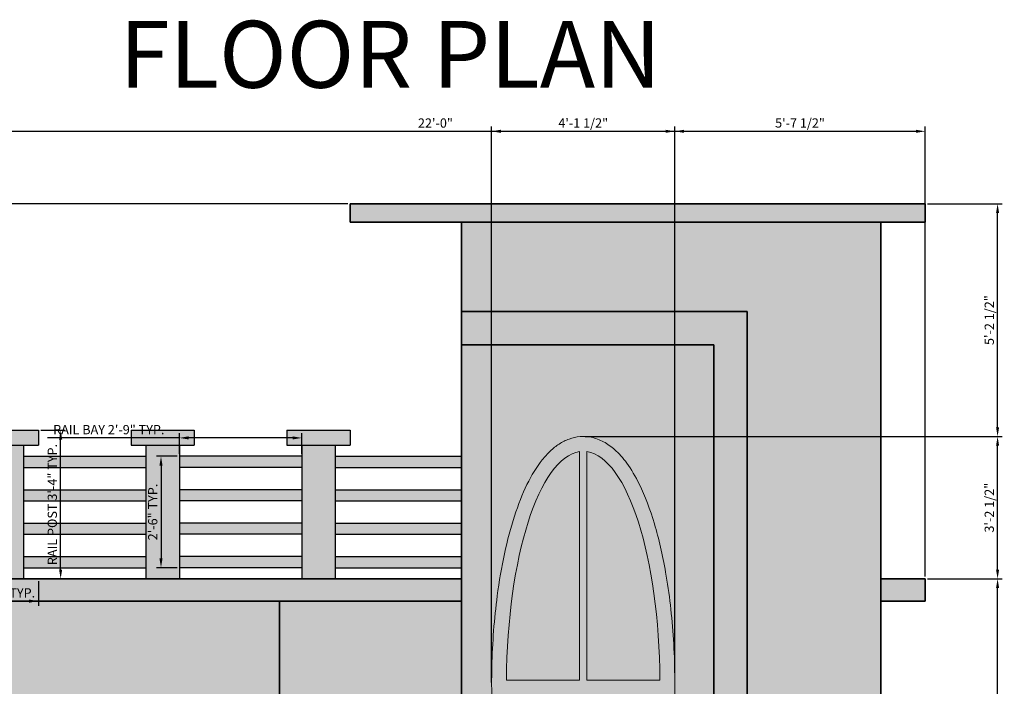
# Model space of a CAD drawing. Units: inches. Extents: x 2150 to 10686, y 1035 to 5077.
# Tile 7 of 12: x 6249 to 6514, y 4425 to 4604. Entities that reach past the tile are written whole.
import ezdxf

# ---------------------------------------------------------------- set-up
doc = ezdxf.new("R2010")
doc.units = ezdxf.units.IN
for name, color, linetype, lineweight in [('A-ANNO-DIMS', 2, 'Continuous', 18), ('A-ANNO-TITL', 3, 'Continuous', 35), ('A-ELEV', 7, 'Continuous', 35), ('A-ELEV-GLAZ', 7, 'Continuous', 18), ('A-ELEV-METL-PATT', 252, 'Continuous', 13), ('A-ELEV-RAIL', 7, 'Continuous', 25)]:
    doc.layers.add(name, color=color, linetype=linetype, lineweight=lineweight)
for name, color, linetype, lineweight, true_color in [('A-ELEV-CONC-PATT', 253, 'Continuous', 13, 0xb2a88f), ('A-ELEV-GLAZ-PATT', 141, 'Continuous', 13, 0xadddf7), ('A-ELEV-PATT', 253, 'Continuous', 13, 0xa5adc8), ('A-ELEV-TRIM-PATT', 85, 'Continuous', 13, 0x58ba48)]:
    doc.layers.add(name, color=color, linetype=linetype, lineweight=lineweight, true_color=true_color)
doc.styles.get("Standard").update_dxf_attribs({"font": 'arial.ttf'})
doc.dimstyles.new('ISO-25', dxfattribs={"dimtxt": 2.5, "dimasz": 2.5, "dimexe": 1.25, "dimexo": 0.625, "dimtad": 1, "dimdec": 0, "dimlunit": 3, "dimtxsty": 'Standard', "dimcen": 2.5, "dimadec": 0, "dimazin": 0, "dimtfac": 1, "dimtdec": 0, "dimtmove": 0, "dimatfit": 3, "dimfxl": 1, "dimarcsym": 0})

# ---------------------------------------------------------------- blocks, each defined once
blk = doc.blocks.new('RAIL-POST-CAPPED')
for p, q in [((-0.0003365621996636, 40.00046013132214), (16.99966343779943, 40.00046013132305)), ((-0.0003365621996636, 40.00046013132214), (-0.0003365621996636, 36.00046013132124)), ((16.99966343779943, 40.00046013132214), (16.99966343780124, 36.00046013132124)), ((-0.0003365621996636, 36.00046013132124), (16.99966343780124, 36.00046013132124)), ((3.999663437800336, 36.00046013132214), (3.999663437800336, 0.0004601313230523)), ((12.99966343780033, 36.00046013132214), (12.99966343780033, 0.0004601313230523))]:
    blk.add_line(p, q)
blk = doc.blocks.new('RAIL-BAY-33IN')
for p, q in [((-0.0003365621996636, 30.00046013132215), (32.99966343780034, 30.00046013132305)), ((-0.0003365621996636, 27.00046013132214), (32.99966343780034, 27.00046013132305)), ((-0.0003365621996636, 21.00046013132305), (32.99966343780034, 21.00046013132214)), ((-0.0003365621996636, 18.00046013132305), (32.99966343780034, 18.00046013132305)), ((-0.0003365621996636, 12.00046013132214), (32.99966343780034, 12.00046013132214)), ((-0.0003365621996636, 9.000460131323052), (32.99966343780034, 9.000460131323052)), ((-0.0003365621996636, 3.000460131323052), (32.99966343780034, 3.000460131323961)), ((-0.0003365621996636, 0.0004601313230523), (32.99966343780034, 0.0004601313239618))]:
    blk.add_line(p, q)
blk = doc.blocks.new('*D64')
at = {"layer": 'A-ANNO-DIMS', "color": 0, "lineweight": -2, "transparency": 16777216}
for p, q in [((6254.232663437805, 4493.484460131325), (6260.857663437809, 4493.484460131325)), ((6259.607663437808, 4455.984460131324), (6259.607663437808, 4490.984460131325)), ((6254.232663437805, 4453.484460131325), (6260.857663437809, 4453.484460131325))]:
    blk.add_line(p, q, dxfattribs=at)
at = {"layer": 'A-ANNO-DIMS', "color": 0, "transparency": 16777216}
for points in [[(6259.190996771142, 4490.984460131325), (6260.024330104475, 4490.984460131325), (6259.607663437808, 4493.484460131325)], [(6259.190996771142, 4455.984460131324), (6260.024330104475, 4455.984460131324), (6259.607663437808, 4453.484460131325)]]:
    blk.add_solid(points, dxfattribs=at)
at = {"layer": 'Defpoints', "color": 0, "transparency": 16777216}
for p in [(6253.607663437805, 4493.484460131325), (6259.607663437808, 4493.484460131325), (6253.607663437805, 4453.484460131325)]:
    blk.add_point(p, dxfattribs=at)
at = {"layer": 'A-ANNO-DIMS', "color": 0, "transparency": 16777216, "insert": (6257.688325102201, 4473.484460131323), "char_height": 2.5, "attachment_point": 5, "rotation": 90}
blk.add_mtext('RAIL POST 3\'-4" TYP.', dxfattribs=at)
blk = doc.blocks.new('*D65')
at = {"layer": 'A-ANNO-DIMS', "color": 0, "lineweight": -2, "transparency": 16777216}
for p, q in [((6236.6076634378, 4452.859460131324), (6236.6076634378, 4446.234460131323)), ((6253.607663437801, 4452.859460131324), (6253.607663437801, 4446.234460131323)), ((6239.107663437801, 4447.484460131323), (6251.107663437801, 4447.484460131323))]:
    blk.add_line(p, q, dxfattribs=at)
at = {"layer": 'A-ANNO-DIMS', "color": 0, "transparency": 16777216}
for points in [[(6239.107663437801, 4447.90112679799), (6239.107663437801, 4447.067793464657), (6236.6076634378, 4447.484460131323)], [(6251.107663437801, 4447.90112679799), (6251.107663437801, 4447.067793464657), (6253.607663437801, 4447.484460131323)]]:
    blk.add_solid(points, dxfattribs=at)
at = {"layer": 'Defpoints', "color": 0, "transparency": 16777216}
for p in [(6236.6076634378, 4453.484460131323), (6253.607663437801, 4453.484460131323), (6253.607663437801, 4447.484460131323)]:
    blk.add_point(p, dxfattribs=at)
at = {"layer": 'A-ANNO-DIMS', "color": 0, "transparency": 16777216, "insert": (6245.1076634378, 4449.385892600627), "char_height": 2.5, "attachment_point": 5}
blk.add_mtext('1\'-5" TYP.', dxfattribs=at)
blk = doc.blocks.new('*D66')
at = {"layer": 'A-ANNO-DIMS', "color": 0, "lineweight": -2, "transparency": 16777216}
for p, q in [((6291.607663437799, 4487.109460131325), (6291.607663437799, 4492.684460131324)), ((6324.6076634378, 4487.109460131325), (6324.6076634378, 4492.684460131324)), ((6291.607663437799, 4491.434460131325), (6256.055139563311, 4491.434460131325)), ((6322.1076634378, 4491.434460131325), (6294.1076634378, 4491.434460131325))]:
    blk.add_line(p, q, dxfattribs=at)
at = {"layer": 'A-ANNO-DIMS', "color": 0, "transparency": 16777216}
for points in [[(6294.1076634378, 4491.851126797992), (6294.1076634378, 4491.017793464658), (6291.607663437799, 4491.434460131325)], [(6322.1076634378, 4491.851126797992), (6322.1076634378, 4491.017793464658), (6324.6076634378, 4491.434460131325)]]:
    blk.add_solid(points, dxfattribs=at)
at = {"layer": 'Defpoints', "color": 0, "transparency": 16777216}
for p in [(6291.607663437799, 4491.434460131325), (6291.607663437799, 4486.484460131324), (6324.6076634378, 4486.484460131324)]:
    blk.add_point(p, dxfattribs=at)
at = {"layer": 'A-ANNO-DIMS', "color": 0, "transparency": 16777216, "insert": (6272.581401500556, 4493.335892600629), "char_height": 2.5, "attachment_point": 5}
blk.add_mtext('RAIL BAY 2\'-9" TYP.', dxfattribs=at)
blk = doc.blocks.new('*D67')
at = {"layer": 'A-ANNO-DIMS', "color": 0, "lineweight": -2, "transparency": 16777216}
for p, q in [((6290.982663437803, 4486.484460131327), (6285.407663437807, 4486.484460131327)), ((6286.657663437807, 4483.984460131327), (6286.657663437807, 4458.984460131327)), ((6290.982663437803, 4456.484460131327), (6285.407663437807, 4456.484460131327))]:
    blk.add_line(p, q, dxfattribs=at)
at = {"layer": 'A-ANNO-DIMS', "color": 0, "transparency": 16777216}
for points in [[(6286.24099677114, 4483.984460131327), (6287.074330104474, 4483.984460131327), (6286.657663437807, 4486.484460131327)], [(6286.24099677114, 4458.984460131327), (6287.074330104474, 4458.984460131327), (6286.657663437807, 4456.484460131327)]]:
    blk.add_solid(points, dxfattribs=at)
at = {"layer": 'Defpoints', "color": 0, "transparency": 16777216}
for p in [(6291.607663437804, 4486.484460131327), (6286.657663437807, 4456.484460131327), (6291.607663437804, 4456.484460131327)]:
    blk.add_point(p, dxfattribs=at)
at = {"layer": 'A-ANNO-DIMS', "color": 0, "transparency": 16777216, "insert": (6284.756230968501, 4471.484460131324), "char_height": 2.5, "attachment_point": 5, "rotation": 90}
blk.add_mtext('2\'-6" TYP.', dxfattribs=at)
blk = doc.blocks.new('*D126')
at = {"layer": 'A-ANNO-DIMS', "color": 0, "lineweight": -2, "transparency": 16777216}
for p, q in [((6228.607663, 4454.10946), (6228.607663, 4575.234459999999)), ((6492.607663, 4454.10946), (6492.607663, 4575.234459999999)), ((6231.107663, 4573.98446), (6490.107663, 4573.98446))]:
    blk.add_line(p, q, dxfattribs=at)
at = {"layer": 'A-ANNO-DIMS', "color": 0, "transparency": 16777216}
for points in [[(6231.107663, 4574.401126666667), (6231.107663, 4573.567793333332), (6228.607663, 4573.98446)], [(6490.107663, 4574.401126666667), (6490.107663, 4573.567793333332), (6492.607663, 4573.98446)]]:
    blk.add_solid(points, dxfattribs=at)
at = {"layer": 'Defpoints', "color": 0, "transparency": 16777216}
for p in [(6492.607663, 4573.98446), (6228.607663, 4453.48446), (6492.607663, 4453.48446)]:
    blk.add_point(p, dxfattribs=at)
at = {"layer": 'A-ANNO-DIMS', "color": 0, "transparency": 16777216, "insert": (6360.607662999999, 4575.885892469304), "char_height": 2.5, "attachment_point": 5}
blk.add_mtext('22\'-0"', dxfattribs=at)
blk = doc.blocks.new('*D127')
at = {"layer": 'A-ANNO-DIMS', "color": 0, "lineweight": -2, "transparency": 16777216}
for p, q in [((6336.982663000004, 4554.484460000002), (6207.857663000007, 4554.484460000002)), ((6209.107663000008, 4292.984460000002), (6209.107663000008, 4551.984460000001)), ((6233.982663000003, 4290.484460000001), (6207.857663000007, 4290.484460000001))]:
    blk.add_line(p, q, dxfattribs=at)
at = {"layer": 'A-ANNO-DIMS', "color": 0, "transparency": 16777216}
for points in [[(6208.69099633334, 4551.984460000001), (6209.524329666674, 4551.984460000001), (6209.107663000008, 4554.484460000002)], [(6208.69099633334, 4292.984460000002), (6209.524329666674, 4292.984460000002), (6209.107663000008, 4290.484460000001)]]:
    blk.add_solid(points, dxfattribs=at)
at = {"layer": 'Defpoints', "color": 0, "transparency": 16777216}
for p in [(6209.107663000008, 4554.484460000002), (6337.607663000003, 4554.484460000002), (6234.607663000003, 4290.484460000001)]:
    blk.add_point(p, dxfattribs=at)
at = {"layer": 'A-ANNO-DIMS', "color": 0, "transparency": 16777216, "insert": (6207.206230530702, 4422.484459999998), "char_height": 2.5, "attachment_point": 5, "rotation": 90}
blk.add_mtext('22\'-0"', dxfattribs=at)
blk = doc.blocks.new('*D128')
at = {"layer": 'A-ANNO-DIMS', "color": 0, "lineweight": -2, "transparency": 16777216}
for p, q in [((6375.761122, 4425.568364), (6375.761122, 4575.234459999999)), ((6425.113627, 4428.198896), (6425.113627, 4575.234459999999)), ((6378.261122, 4573.98446), (6422.613627, 4573.98446))]:
    blk.add_line(p, q, dxfattribs=at)
at = {"layer": 'A-ANNO-DIMS', "color": 0, "transparency": 16777216}
for points in [[(6378.261122, 4574.401126666667), (6378.261122, 4573.567793333332), (6375.761122, 4573.98446)], [(6422.613627, 4574.401126666667), (6422.613627, 4573.567793333332), (6425.113627, 4573.98446)]]:
    blk.add_solid(points, dxfattribs=at)
at = {"layer": 'Defpoints', "color": 0, "transparency": 16777216}
for p in [(6425.113627, 4573.98446), (6425.113627, 4427.573896), (6375.761122, 4424.943363999999)]:
    blk.add_point(p, dxfattribs=at)
at = {"layer": 'A-ANNO-DIMS', "color": 0, "transparency": 16777216, "insert": (6400.4373745, 4575.902093015006), "char_height": 2.5, "attachment_point": 5}
blk.add_mtext('4\'-1 1/2"', dxfattribs=at)
blk = doc.blocks.new('*D129')
at = {"layer": 'A-ANNO-DIMS', "color": 0, "lineweight": -2, "transparency": 16777216}
for p, q in [((6425.113627, 4428.198896), (6425.113627, 4575.234459999999)), ((6492.607663, 4555.109459999999), (6492.607663, 4575.234459999999)), ((6427.613626999999, 4573.98446), (6490.107663, 4573.98446))]:
    blk.add_line(p, q, dxfattribs=at)
at = {"layer": 'A-ANNO-DIMS', "color": 0, "transparency": 16777216}
for points in [[(6427.613626999999, 4574.401126666667), (6427.613626999999, 4573.567793333332), (6425.113627, 4573.98446)], [(6490.107663, 4574.401126666667), (6490.107663, 4573.567793333332), (6492.607663, 4573.98446)]]:
    blk.add_solid(points, dxfattribs=at)
at = {"layer": 'Defpoints', "color": 0, "transparency": 16777216}
for p in [(6492.607663, 4573.98446), (6492.607663, 4554.48446), (6425.113627, 4427.573896)]:
    blk.add_point(p, dxfattribs=at)
at = {"layer": 'A-ANNO-DIMS', "color": 0, "transparency": 16777216, "insert": (6458.860645, 4575.902093015006), "char_height": 2.5, "attachment_point": 5}
blk.add_mtext('5\'-7 1/2"', dxfattribs=at)
blk = doc.blocks.new('*D131')
at = {"layer": 'A-ANNO-DIMS', "color": 0, "lineweight": -2, "transparency": 16777216}
for p, q in [((6493.232663000004, 4453.484460000001), (6513.357663000007, 4453.484460000001)), ((6512.107663000008, 4361.024472000002), (6512.107663000008, 4450.984460000001)), ((6401.069858000004, 4358.524472000001), (6513.357663000007, 4358.524472000001))]:
    blk.add_line(p, q, dxfattribs=at)
at = {"layer": 'A-ANNO-DIMS', "color": 0, "transparency": 16777216}
for points in [[(6511.69099633334, 4450.984460000001), (6512.524329666674, 4450.984460000001), (6512.107663000008, 4453.484460000001)], [(6511.69099633334, 4361.024472000002), (6512.524329666674, 4361.024472000002), (6512.107663000008, 4358.524472000001)]]:
    blk.add_solid(points, dxfattribs=at)
at = {"layer": 'Defpoints', "color": 0, "transparency": 16777216}
for p in [(6492.607663000004, 4453.484460000001), (6512.107663000008, 4453.484460000001), (6400.444858000003, 4358.524472000001)]:
    blk.add_point(p, dxfattribs=at)
at = {"layer": 'A-ANNO-DIMS', "color": 0, "transparency": 16777216, "insert": (6510.227547038205, 4406.004465999998), "char_height": 2.5, "attachment_point": 5, "rotation": 90}
blk.add_mtext('7\'-11"', dxfattribs=at)
blk = doc.blocks.new('*D132')
at = {"layer": 'A-ANNO-DIMS', "color": 0, "lineweight": -2, "transparency": 16777216}
for p, q in [((6400.954167000003, 4491.810058000002), (6513.357663000007, 4491.810058000002)), ((6512.107663000008, 4455.984460000001), (6512.107663000008, 4489.310058000001)), ((6493.232663000004, 4453.484460000001), (6513.357663000007, 4453.484460000001))]:
    blk.add_line(p, q, dxfattribs=at)
at = {"layer": 'A-ANNO-DIMS', "color": 0, "transparency": 16777216}
for points in [[(6511.69099633334, 4489.310058000001), (6512.524329666674, 4489.310058000001), (6512.107663000008, 4491.810058000002)], [(6511.69099633334, 4455.984460000001), (6512.524329666674, 4455.984460000001), (6512.107663000008, 4453.484460000001)]]:
    blk.add_solid(points, dxfattribs=at)
at = {"layer": 'Defpoints', "color": 0, "transparency": 16777216}
for p in [(6400.329167000004, 4491.810058000002), (6512.107663000008, 4491.810058000002), (6492.607663000004, 4453.484460000001)]:
    blk.add_point(p, dxfattribs=at)
at = {"layer": 'A-ANNO-DIMS', "color": 0, "transparency": 16777216, "insert": (6510.189177324699, 4472.647258999999), "char_height": 2.5, "attachment_point": 5, "rotation": 90}
blk.add_mtext('3\'-2 1/2"', dxfattribs=at)
blk = doc.blocks.new('*D133')
at = {"layer": 'A-ANNO-DIMS', "color": 0, "lineweight": -2, "transparency": 16777216}
for p, q in [((6493.232663000004, 4554.484460000002), (6513.357663000007, 4554.484460000002)), ((6512.107663000008, 4494.310058000002), (6512.107663000008, 4551.984460000001)), ((6400.954167000003, 4491.810058000002), (6513.357663000007, 4491.810058000002))]:
    blk.add_line(p, q, dxfattribs=at)
at = {"layer": 'A-ANNO-DIMS', "color": 0, "transparency": 16777216}
for points in [[(6511.69099633334, 4551.984460000001), (6512.524329666674, 4551.984460000001), (6512.107663000008, 4554.484460000002)], [(6511.69099633334, 4494.310058000002), (6512.524329666674, 4494.310058000002), (6512.107663000008, 4491.810058000002)]]:
    blk.add_solid(points, dxfattribs=at)
at = {"layer": 'Defpoints', "color": 0, "transparency": 16777216}
for p in [(6492.607663000004, 4554.484460000002), (6512.107663000008, 4554.484460000002), (6400.329167000004, 4491.810058000002)]:
    blk.add_point(p, dxfattribs=at)
at = {"layer": 'A-ANNO-DIMS', "color": 0, "transparency": 16777216, "insert": (6510.190029985, 4523.147258999999), "char_height": 2.5, "attachment_point": 5, "rotation": 90}
blk.add_mtext('5\'-2 1/2"', dxfattribs=at)

msp = doc.modelspace()

# ---------------------------------------------------------------- hatches: boundary and pattern name
at = {"layer": 'A-ELEV-CONC-PATT'}
h = msp.add_hatch(dxfattribs=at)
h.set_pattern_fill('AR-CONC', color=256, scale=0.02)
h.set_pattern_definition([(50, (0, 0), (3.64369337992008, -0.3187817107780617), [0.381, -4.191]), (355, (0, 0), (-0.7048684284993869, 3.821136904780702), [0.3048, -3.3528116834]), (100.4514447, (0.30364014, -0.02656507), (2.938824941807065, 3.502355038243901), [0.323800176, -3.561804891999999]), (46.18420000000001, (0, 1.016), (5.421580817842598, -0.8408465586545428), [0.5714999999999999, -6.286499999999999]), (96.63555760999996, (0.4517980000000001, 0.94593), (4.74808268103006, 4.94852249195443), [0.4857004628000001, -5.342712163199999]), (351.18415117, (0, 1.016), (4.74808268129954, 4.948522491710653), [0.4571993414000001, -5.029194638399999]), (21, (0.508, 0.762), (3.032287825382649, -2.045303963741752), [0.381, -4.191]), (326, (0.508, 0.762), (1.236040566952941, 3.683759322446385), [0.3048, -3.352799999999999]), (71.45144499999999, (0.760690652, 0.5915580020000001), (4.268328385574323, 1.638455377718104), [0.323800176, -3.561798751999999]), (37.5, (0, 0), (0.0617720650118363, 1.691100777463062), [0, -3.312159999999999, 0, -3.4036, 0, -3.3655]), (7.499999999999999, (0, 0), (1.336393250206114, 2.00361149636239), [0, -1.940559999999999, 0, -3.235959999999999, 0, -1.2827]), (327.5, (-1.132839999999999, 0), (2.711811903337427, -0.1145748798534689), [0, -1.27, 0, -3.9624, 0, -5.257799999999999]), (317.5, (-1.64084, 0), (2.962583627720361, 0.5085298206666607), [0, -1.650999999999999, 0, -2.63144, 0, -3.7338])])
h.paths.add_polyline_path([(6444.633239304355, 4525.484460131322), (6367.6076634378, 4525.484460131324), (6367.6076634378, 4516.484460131324), (6435.633239304355, 4516.484460131323), (6435.633239304355, 4303.484460131323), (6444.633239304355, 4303.484460131323)])
h.paths.add_polyline_path([(6367.6076634378, 4453.484460131323), (6228.6076634378, 4453.484460131323), (6228.6076634378, 4447.484460131323), (6367.6076634378, 4447.484460131323)])
h.paths.add_polyline_path([(6492.607663437801, 4453.484460131323), (6480.633239304353, 4453.484460131322), (6480.633239304353, 4447.484460131323), (6492.607663437801, 4447.484460131323)])
h.paths.add_polyline_path([(6492.607663437801, 4554.484460131323), (6337.6076634378, 4554.484460131323), (6337.607663437799, 4549.484460131323), (6492.607663437799, 4549.484460131323)])
at = {"layer": 'A-ELEV-GLAZ-PATT'}
h = msp.add_hatch(color=256, dxfattribs=at)
h.dxf.hatch_style = 1
h.paths.add_polyline_path([(6279.607663437801, 4384.484460131323), (6267.607663437801, 4384.484460131323), (6267.6076634378, 4372.484460131324), (6279.607663437801, 4372.484460131324)])
h.paths.add_polyline_path([(6291.607663437801, 4384.484460131323), (6279.607663437801, 4384.484460131323), (6279.607663437801, 4372.484460131324), (6291.607663437801, 4372.484460131324)])
edge = h.paths.add_edge_path()
edge.add_ellipse((6400.444858416264, 4425.167712730096), major_axis=(0, -62.64324057997146), ratio=0.3301887017017349, start_angle=180.9156291084783, end_angle=267.2317619230999)
edge.add_line((6379.76340377621, 4426.167712730096), (6399.444858416265, 4426.167712730096))
edge.add_line((6399.444858416265, 4426.167712730096), (6399.444858416265, 4487.737700317675))
edge = h.paths.add_edge_path()
edge.add_ellipse((6400.444858416264, 4425.167712730096), major_axis=(0, -62.64324057997146), ratio=0.3301887017017349, start_angle=452.7682380769, end_angle=539.0843708915216)
edge.add_line((6401.444858416265, 4487.737700317675), (6401.444858416265, 4426.167712730096))
edge.add_line((6401.444858416265, 4426.167712730096), (6421.126313056319, 4426.167712730096))
edge = h.paths.add_edge_path()
edge.add_ellipse((6400.444858416264, 4425.167712730096), major_axis=(0, -62.64324057997146), ratio=0.3301887017017349, start_angle=378.88994340641, end_angle=447.2317619231)
edge.add_line((6421.126313056319, 4424.167712730096), (6401.444858416265, 4424.167712730096))
edge.add_line((6401.444858416265, 4424.167712730096), (6401.444858416265, 4376.02078865707))
edge.add_line((6401.444858416265, 4376.02078865707), (6408.633239304354, 4376.02078865707))
edge.add_line((6408.633239304354, 4376.02078865707), (6408.633239304354, 4382.020788657071))
edge.add_line((6408.633239304354, 4382.020788657071), (6415.329204846509, 4381.669182122283))
edge = h.paths.add_edge_path()
edge.add_line((6399.444858416265, 4424.167712730096), (6379.76340377621, 4424.167712730096))
edge.add_ellipse((6400.444858416264, 4425.167712730096), major_axis=(0, -62.64324057997146), ratio=0.3301887017017349, start_angle=272.7682380768999, end_angle=349.9116256040723)
edge.add_line((6390.633239304354, 4370.020788657071), (6399.444858416265, 4370.020788657071))
edge.add_line((6399.444858416265, 4370.020788657071), (6399.444858416265, 4424.167712730096))
edge = h.paths.add_edge_path()
edge.add_line((6399.444858416265, 4370.020788657071), (6390.633239304354, 4370.020788657071))
edge.add_ellipse((6400.444858416264, 4425.167712730096), major_axis=(0, -62.64324057997146), ratio=0.3301887017017349, start_angle=349.9116256040723, end_angle=359.0843708915216)
edge.add_line((6399.444858416265, 4362.597725142516), (6399.444858416265, 4370.020788657071))
edge = h.paths.add_edge_path()
edge.add_ellipse((6400.444858416264, 4425.167712730096), major_axis=(0, -62.64324057997146), ratio=0.3301887017017349, start_angle=360.9156291084783, end_angle=378.88994340641)
edge.add_line((6415.329204846509, 4381.669182122283), (6408.633239304354, 4382.020788657071))
edge.add_line((6408.633239304354, 4382.020788657071), (6408.633239304354, 4376.02078865707))
edge.add_line((6408.633239304354, 4376.02078865707), (6401.444858416265, 4376.02078865707))
edge.add_line((6401.444858416265, 4376.02078865707), (6401.444858416265, 4362.597725142516))
at = {"layer": 'A-ELEV-METL-PATT'}
h = msp.add_hatch(color=256, dxfattribs=at)
h.dxf.hatch_style = 1
h.paths.add_polyline_path([(6253.6076634378, 4493.484460131323), (6236.6076634378, 4493.484460131322), (6236.6076634378, 4489.484460131321), (6253.607663437801, 4489.484460131321)])
h.paths.add_polyline_path([(6295.607663437801, 4493.484460131323), (6278.6076634378, 4493.484460131323), (6278.6076634378, 4489.484460131322), (6295.607663437801, 4489.484460131325)])
h.paths.add_polyline_path([(6337.6076634378, 4493.484460131323), (6320.607663437801, 4493.484460131324), (6320.607663437801, 4489.484460131322), (6337.6076634378, 4489.484460131318)])
h = msp.add_hatch(color=256, dxfattribs=at)
h.dxf.hatch_style = 1
edge = h.paths.add_edge_path()
edge.add_spline(control_points=[(6400.444858416264, 4358.524472150125), (6401.486440814489, 4358.524472150125), (6402.526505044808, 4358.677401357236), (6404.522486905328, 4359.255063234454), (6405.478003331038, 4359.677509034017), (6407.281736042183, 4360.731176144923), (6408.131339490663, 4361.361806443027), (6409.740207013673, 4362.793659380537), (6410.500149994661, 4363.595296803934), (6412.700838569434, 4366.265752912591), (6414.03394570237, 4368.379499630626), (6416.487744706213, 4373.197243253772), (6417.606172835956, 4375.903063890813), (6419.631029857393, 4381.840607040826), (6420.536486327513, 4385.072192199597), (6422.117938633519, 4391.962202533656), (6422.793588111736, 4395.620342382234), (6424.200323950252, 4405.332886237875), (6424.756775730746, 4411.600724829638), (6425.233072301224, 4424.345165291339), (6425.152698848673, 4430.819672112305), (6424.360861114452, 4443.427756971612), (6423.649784349251, 4449.559211921115), (6421.832101343849, 4459.914160022554), (6420.824100186611, 4464.280479948769), (6418.459699862937, 4472.224057176997), (6417.105531965493, 4475.800577784561), (6414.530984821721, 4481.046021704659), (6413.400413444257, 4482.963765924061), (6411.159609652, 4486.022314366695), (6410.081239671351, 4487.242292157316), (6407.981904490796, 4489.103336574784), (6406.994481886034, 4489.812440503778), (6404.88004816331, 4490.945334575583), (6403.750412373089, 4491.367263683768), (6401.591707320996, 4491.795744529485), (6400.578062848126, 4491.856564882596), (6398.574329452856, 4491.695615966483), (6397.586567833659, 4491.47475953499), (6395.700279883302, 4490.794741309719), (6394.801423289315, 4490.337316033343), (6393.101630982474, 4489.237707960262), (6392.299575991901, 4488.59571921333), (6390.776032761522, 4487.156246990203), (6390.054097434259, 4486.358390989495), (6387.868726596746, 4483.603993381065), (6386.519519142056, 4481.381571183187), (6384.042618140686, 4476.318979222956), (6382.917389359787, 4473.477169667343), (6380.892123096994, 4467.249882245213), (6379.993066323842, 4463.864616669574), (6378.439918554827, 4456.661812920038), (6377.786169577303, 4452.844597947903), (6376.462930365054, 4442.788115239438), (6375.974391004774, 4436.347147441612), (6375.659764204387, 4423.32378833974), (6375.833828926627, 4416.743682061819), (6376.8313878542, 4404.020783955098), (6377.654325200822, 4397.880344812312), (6379.642069279475, 4387.821914067098), (6380.689035460468, 4383.713325470128), (6383.106877716371, 4376.272307259607), (6384.47532253611, 4372.940336073535), (6387.048331366607, 4368.105027158752), (6388.164220640812, 4366.356485480582), (6390.369702204264, 4363.581332383819), (6391.427944586487, 4362.479757644216), (6393.496381316636, 4360.802633777571), (6394.475915167926, 4360.166036636088), (6396.563807655099, 4359.173441496676), (6397.674090126379, 4358.819701830231), (6399.355629057865, 4358.565786838256), (6399.900211293723, 4358.524472150125), (6400.444858416264, 4358.524472150125)], knot_values=[0, 0, 0, 0, 0.0952714022776172, 0.0952714022776172, 0.1905428045552344, 0.1905428045552344, 0.2858142068328516, 0.2858142068328516, 0.3810856091104688, 0.3810856091104688, 0.575169634462188, 0.575169634462188, 0.7692536598139071, 0.7692536598139071, 0.9633376851656262, 0.9633376851656262, 1.157421710517345, 1.157421710517345, 1.458089536658081, 1.458089536658081, 1.758757362798818, 1.758757362798818, 2.059425188939554, 2.059425188939554, 2.304413142887573, 2.304413142887573, 2.549401096835591, 2.549401096835591, 2.718168677128249, 2.718168677128249, 2.856837524264077, 2.856837524264077, 2.966492349551455, 2.966492349551455, 3.076147174838833, 3.076147174838833, 3.168108685177037, 3.168108685177037, 3.260070195515242, 3.260070195515242, 3.352031705853447, 3.352031705853447, 3.443993216191651, 3.443993216191651, 3.535954726529856, 3.535954726529856, 3.735259798893268, 3.735259798893268, 3.93456487125668, 3.93456487125668, 4.133869943620092, 4.133869943620092, 4.333175015983504, 4.333175015983504, 4.639352924429541, 4.639352924429541, 4.945530832875578, 4.945530832875578, 5.251708741321616, 5.251708741321616, 5.489766878495931, 5.489766878495931, 5.727825015670246, 5.727825015670246, 5.88940932659502, 5.88940932659502, 6.02159730311115, 6.02159730311115, 6.127482428421133, 6.127482428421133, 6.233367553731117, 6.233367553731117, 6.283185307179586, 6.283185307179586, 6.283185307179586, 6.283185307179586], degree=3, periodic=0)
edge = h.paths.add_edge_path(flags=16)
edge.add_line((6399.444858416265, 4487.737700317675), (6399.444858416265, 4426.167712730096))
edge.add_line((6399.444858416265, 4426.167712730096), (6379.76340377621, 4426.167712730096))
edge.add_ellipse((6400.444858416264, 4425.167712730096), major_axis=(0, -62.64324057997146), ratio=0.3301887017017349, start_angle=180.9156291084783, end_angle=267.2317619230999, ccw=False)
edge = h.paths.add_edge_path(flags=16)
edge.add_ellipse((6400.444858416264, 4425.167712730096), major_axis=(0, -62.64324057997146), ratio=0.3301887017017349, start_angle=452.7682380769001, end_angle=539.0843708915218, ccw=False)
edge.add_line((6421.126313056319, 4426.167712730096), (6401.444858416265, 4426.167712730096))
edge.add_line((6401.444858416265, 4426.167712730096), (6401.444858416265, 4487.737700317675))
edge = h.paths.add_edge_path(flags=16)
edge.add_line((6399.444858416265, 4424.167712730097), (6399.444858416265, 4370.020788657071))
edge.add_line((6399.444858416265, 4370.020788657071), (6399.633239304353, 4370.020788657071))
edge.add_line((6399.633239304353, 4370.020788657071), (6399.633239304353, 4376.02078865707))
edge.add_line((6399.633239304353, 4376.02078865707), (6401.444858416265, 4376.02078865707))
edge.add_line((6401.444858416265, 4376.02078865707), (6401.444858416265, 4424.167712730096))
edge.add_line((6401.444858416265, 4424.167712730096), (6421.126313056319, 4424.167712730096))
edge.add_ellipse((6400.444858416264, 4425.167712730096), major_axis=(0, -62.64324057997146), ratio=0.3301887017017349, start_angle=378.88994340641005, end_angle=447.23176192310007, ccw=False)
edge.add_ellipse((6400.444858416264, 4425.167712730096), major_axis=(0, -62.64324057997146), ratio=0.3301887017017349, start_angle=360.9156291084783, end_angle=378.88994340641005, ccw=False)
edge.add_line((6401.444858416265, 4362.597725142516), (6401.444858416265, 4376.02078865707))
edge.add_line((6401.444858416265, 4376.02078865707), (6399.633239304353, 4376.02078865707))
edge.add_line((6399.633239304353, 4376.02078865707), (6399.633239304353, 4370.020788657071))
edge.add_line((6399.633239304353, 4370.020788657071), (6399.444858416265, 4370.020788657071))
edge.add_line((6399.444858416265, 4370.020788657071), (6399.444858416265, 4362.597725142516))
edge.add_ellipse((6400.444858416264, 4425.167712730096), major_axis=(0, -62.64324057997146), ratio=0.3301887017017349, start_angle=349.9116256040723, end_angle=359.0843708915217, ccw=False)
edge.add_ellipse((6400.444858416264, 4425.167712730096), major_axis=(0, -62.64324057997146), ratio=0.3301887017017349, start_angle=272.76823807689993, end_angle=349.9116256040723, ccw=False)
edge.add_line((6379.76340377621, 4424.167712730096), (6399.444858416265, 4424.167712730097))
h.paths.add_polyline_path([(6294.607663437801, 4387.484460131323), (6264.6076634378, 4387.484460131323), (6264.6076634378, 4369.484460131324), (6294.607663437801, 4369.484460131324)])
h.paths.add_polyline_path([(6267.607663437801, 4384.484460131323), (6291.607663437801, 4384.484460131323), (6291.607663437801, 4372.484460131324), (6267.6076634378, 4372.484460131324)], flags=16)
h = msp.add_hatch(color=256, dxfattribs=at)
h.dxf.hatch_style = 1
h.paths.add_polyline_path([(6282.607663437801, 4486.484460131324), (6249.6076634378, 4486.484460131322), (6249.6076634378, 4483.484460131323), (6282.607663437801, 4483.484460131323)])
h.paths.add_polyline_path([(6324.607663437801, 4486.484460131324), (6291.607663437801, 4486.484460131324), (6291.607663437801, 4483.484460131323), (6324.607663437801, 4483.484460131323)])
h.paths.add_polyline_path([(6367.6076634378, 4486.484460131324), (6333.607663437801, 4486.484460131324), (6333.607663437801, 4483.484460131323), (6367.6076634378, 4483.484460131323)])
h.paths.add_polyline_path([(6367.6076634378, 4477.484460131323), (6333.607663437801, 4477.484460131323), (6333.607663437801, 4474.484460131323), (6367.6076634378, 4474.484460131323)])
h.paths.add_polyline_path([(6367.6076634378, 4468.484460131324), (6333.607663437801, 4468.484460131322), (6333.607663437801, 4465.484460131324), (6367.6076634378, 4465.484460131324)])
h.paths.add_polyline_path([(6367.6076634378, 4459.484460131323), (6333.607663437801, 4459.484460131323), (6333.607663437801, 4456.484460131323), (6367.6076634378, 4456.484460131323)])
h.paths.add_polyline_path([(6324.607663437801, 4459.484460131323), (6291.607663437801, 4459.484460131323), (6291.607663437801, 4456.484460131324), (6324.607663437801, 4456.484460131323)])
h.paths.add_polyline_path([(6324.607663437801, 4468.484460131322), (6291.607663437801, 4468.484460131322), (6291.607663437801, 4465.484460131324), (6324.607663437801, 4465.484460131324)])
h.paths.add_polyline_path([(6324.607663437801, 4477.484460131323), (6291.607663437801, 4477.484460131322), (6291.607663437801, 4474.484460131323), (6324.607663437801, 4474.484460131323)])
h.paths.add_polyline_path([(6282.607663437801, 4477.484460131322), (6249.6076634378, 4477.484460131323), (6249.6076634378, 4474.484460131323), (6282.607663437801, 4474.484460131323)])
h.paths.add_polyline_path([(6282.607663437801, 4468.484460131322), (6249.6076634378, 4468.484460131322), (6249.6076634378, 4465.484460131324), (6282.607663437801, 4465.484460131324)])
h.paths.add_polyline_path([(6282.607663437801, 4459.484460131323), (6249.6076634378, 4459.484460131323), (6249.6076634378, 4456.484460131323), (6282.607663437801, 4456.484460131324)])
at = {"layer": 'A-ELEV-PATT'}
h = msp.add_hatch(color=256, dxfattribs=at)
h.dxf.hatch_style = 1
h.paths.add_polyline_path([(6435.633239304355, 4516.484460131323), (6367.6076634378, 4516.484460131324), (6367.6076634378, 4303.484460131323), (6435.633239304355, 4303.484460131323)])
edge = h.paths.add_edge_path(flags=16)
edge.add_spline(control_points=[(6400.444858416264, 4358.524472150125), (6401.486440814489, 4358.524472150125), (6402.526505044808, 4358.677401357236), (6404.522486905328, 4359.255063234454), (6405.478003331038, 4359.677509034017), (6407.281736042183, 4360.731176144923), (6408.131339490663, 4361.361806443027), (6409.740207013673, 4362.793659380537), (6410.500149994661, 4363.595296803934), (6412.700838569434, 4366.265752912591), (6414.03394570237, 4368.379499630626), (6416.487744706213, 4373.197243253772), (6417.606172835956, 4375.903063890813), (6419.631029857393, 4381.840607040826), (6420.536486327513, 4385.072192199597), (6422.117938633519, 4391.962202533656), (6422.793588111736, 4395.620342382234), (6424.200323950252, 4405.332886237875), (6424.756775730746, 4411.600724829638), (6425.233072301224, 4424.345165291339), (6425.152698848673, 4430.819672112305), (6424.360861114452, 4443.427756971612), (6423.649784349251, 4449.559211921115), (6421.832101343849, 4459.914160022554), (6420.824100186611, 4464.280479948769), (6418.459699862937, 4472.224057176997), (6417.105531965493, 4475.800577784561), (6414.530984821721, 4481.046021704659), (6413.400413444257, 4482.963765924061), (6411.159609652, 4486.022314366695), (6410.081239671351, 4487.242292157316), (6407.981904490796, 4489.103336574784), (6406.994481886034, 4489.812440503778), (6404.88004816331, 4490.945334575583), (6403.750412373089, 4491.367263683768), (6401.591707320996, 4491.795744529485), (6400.578062848126, 4491.856564882596), (6398.574329452856, 4491.695615966483), (6397.586567833659, 4491.47475953499), (6395.700279883302, 4490.794741309719), (6394.801423289315, 4490.337316033343), (6393.101630982474, 4489.237707960262), (6392.299575991901, 4488.59571921333), (6390.776032761522, 4487.156246990203), (6390.054097434259, 4486.358390989495), (6387.868726596746, 4483.603993381065), (6386.519519142056, 4481.381571183187), (6384.042618140686, 4476.318979222956), (6382.917389359787, 4473.477169667343), (6380.892123096994, 4467.249882245213), (6379.993066323842, 4463.864616669574), (6378.439918554827, 4456.661812920038), (6377.786169577303, 4452.844597947903), (6376.462930365054, 4442.788115239438), (6375.974391004774, 4436.347147441612), (6375.659764204387, 4423.32378833974), (6375.833828926627, 4416.743682061819), (6376.8313878542, 4404.020783955098), (6377.654325200822, 4397.880344812312), (6379.642069279475, 4387.821914067098), (6380.689035460468, 4383.713325470128), (6383.106877716371, 4376.272307259607), (6384.47532253611, 4372.940336073535), (6387.048331366607, 4368.105027158752), (6388.164220640812, 4366.356485480582), (6390.369702204264, 4363.581332383819), (6391.427944586487, 4362.479757644216), (6393.496381316636, 4360.802633777571), (6394.475915167926, 4360.166036636088), (6396.563807655099, 4359.173441496676), (6397.674090126379, 4358.819701830231), (6399.355629057865, 4358.565786838256), (6399.900211293723, 4358.524472150125), (6400.444858416264, 4358.524472150125)], knot_values=[0, 0, 0, 0, 0.0952714022776172, 0.0952714022776172, 0.1905428045552344, 0.1905428045552344, 0.2858142068328516, 0.2858142068328516, 0.3810856091104688, 0.3810856091104688, 0.575169634462188, 0.575169634462188, 0.7692536598139071, 0.7692536598139071, 0.9633376851656262, 0.9633376851656262, 1.157421710517345, 1.157421710517345, 1.458089536658081, 1.458089536658081, 1.758757362798818, 1.758757362798818, 2.059425188939554, 2.059425188939554, 2.304413142887573, 2.304413142887573, 2.549401096835591, 2.549401096835591, 2.718168677128249, 2.718168677128249, 2.856837524264077, 2.856837524264077, 2.966492349551455, 2.966492349551455, 3.076147174838833, 3.076147174838833, 3.168108685177037, 3.168108685177037, 3.260070195515242, 3.260070195515242, 3.352031705853447, 3.352031705853447, 3.443993216191651, 3.443993216191651, 3.535954726529856, 3.535954726529856, 3.735259798893268, 3.735259798893268, 3.93456487125668, 3.93456487125668, 4.133869943620092, 4.133869943620092, 4.333175015983504, 4.333175015983504, 4.639352924429541, 4.639352924429541, 4.945530832875578, 4.945530832875578, 5.251708741321616, 5.251708741321616, 5.489766878495931, 5.489766878495931, 5.727825015670246, 5.727825015670246, 5.88940932659502, 5.88940932659502, 6.02159730311115, 6.02159730311115, 6.127482428421133, 6.127482428421133, 6.233367553731117, 6.233367553731117, 6.283185307179586, 6.283185307179586, 6.283185307179586, 6.283185307179586], degree=3, periodic=0)
edge = h.paths.add_edge_path(flags=0)
edge.add_ellipse((6400.444858416264, 4425.167712730096), major_axis=(0, -62.64324057997146), ratio=0.3301887017017349, start_angle=452.7682380769001, end_angle=539.0843708915218, ccw=False)
edge.add_line((6421.126313056319, 4426.167712730096), (6401.444858416265, 4426.167712730096))
edge.add_line((6401.444858416265, 4426.167712730096), (6401.444858416265, 4487.737700317675))
edge = h.paths.add_edge_path(flags=0)
edge.add_line((6399.444858416265, 4487.737700317675), (6399.444858416265, 4426.167712730096))
edge.add_line((6399.444858416265, 4426.167712730096), (6379.76340377621, 4426.167712730096))
edge.add_ellipse((6400.444858416264, 4425.167712730096), major_axis=(0, -62.64324057997146), ratio=0.3301887017017349, start_angle=180.9156291084783, end_angle=267.2317619230999, ccw=False)
edge = h.paths.add_edge_path(flags=0)
edge.add_ellipse((6400.444858416264, 4425.167712730096), major_axis=(0, -62.64324057997146), ratio=0.3301887017017349, start_angle=378.88994340641005, end_angle=447.23176192310007, ccw=False)
edge.add_ellipse((6400.444858416264, 4425.167712730096), major_axis=(0, -62.64324057997146), ratio=0.3301887017017349, start_angle=360.9156291084783, end_angle=378.88994340641005, ccw=False)
edge.add_line((6401.444858416265, 4362.597725142516), (6401.444858416265, 4376.02078865707))
edge.add_line((6401.444858416265, 4376.02078865707), (6399.633239304353, 4376.02078865707))
edge.add_line((6399.633239304353, 4376.02078865707), (6399.633239304353, 4370.020788657071))
edge.add_line((6399.633239304353, 4370.020788657071), (6399.444858416265, 4362.597725142516))
edge.add_ellipse((6400.444858416264, 4425.167712730096), major_axis=(0, -62.64324057997146), ratio=0.3301887017017349, start_angle=349.9116256040723, end_angle=359.0843708915217, ccw=False)
edge.add_ellipse((6400.444858416264, 4425.167712730096), major_axis=(0, -62.64324057997146), ratio=0.3301887017017349, start_angle=272.76823807689993, end_angle=349.9116256040723, ccw=False)
edge.add_line((6379.76340377621, 4424.167712730096), (6399.444858416265, 4424.167712730096))
edge.add_line((6399.444858416265, 4424.167712730096), (6399.444858416265, 4376.02078865707))
edge.add_line((6399.444858416265, 4376.02078865707), (6401.444858416265, 4376.02078865707))
edge.add_line((6401.444858416265, 4376.02078865707), (6401.444858416265, 4424.167712730096))
edge.add_line((6401.444858416265, 4424.167712730096), (6421.126313056319, 4424.167712730096))
h = msp.add_hatch(color=256, dxfattribs=at)
h.dxf.hatch_style = 1
h.paths.add_polyline_path([(6318.6076634378, 4447.484460131323), (6240.6076634378, 4447.484460131323), (6240.6076634378, 4303.484460131323), (6318.607663437799, 4303.484460131323)])
h.paths.add_polyline_path([(6294.607663437801, 4387.484460131323), (6294.607663437801, 4369.484460131324), (6264.6076634378, 4369.484460131324), (6264.6076634378, 4387.484460131323)], flags=16)
h.paths.add_polyline_path([(6291.607663437801, 4384.484460131324), (6291.607663437801, 4372.484460131324), (6267.6076634378, 4372.484460131324), (6267.607663437801, 4384.484460131323)], flags=0)
h = msp.add_hatch(color=256, dxfattribs=at)
h.dxf.hatch_style = 1
h.paths.add_polyline_path([(6367.6076634378, 4447.484460131323), (6318.6076634378, 4447.484460131323), (6318.607663437799, 4303.484460131323), (6319.607663437792, 4303.484460131323), (6319.607663437802, 4387.484460131323), (6355.607663437799, 4387.484460131323), (6355.607663437799, 4363.484460131324), (6366.607663437799, 4363.484460131324), (6366.6076634378, 4305.484460131324), (6320.6076634378, 4305.484460131324), (6320.6076634378, 4303.484460131323), (6367.6076634378, 4303.484460131323)])
at = {"layer": 'A-ELEV-TRIM-PATT'}
h = msp.add_hatch(color=256, dxfattribs=at)
h.dxf.hatch_style = 1
h.paths.add_polyline_path([(6480.633239304353, 4549.484460131323), (6367.6076634378, 4549.484460131323), (6367.6076634378, 4525.484460131324), (6444.633239304355, 4525.484460131322), (6444.633239304355, 4303.484460131323), (6480.633239304355, 4303.484460131323)])
h = msp.add_hatch(color=256, dxfattribs=at)
h.dxf.hatch_style = 1
h.paths.add_polyline_path([(6249.6076634378, 4489.484460131321), (6240.6076634378, 4489.484460131321), (6240.6076634378, 4453.484460131323), (6249.6076634378, 4453.484460131323)])
h.paths.add_polyline_path([(6291.607663437801, 4489.484460131325), (6282.607663437801, 4489.484460131324), (6282.607663437801, 4453.484460131323), (6291.607663437801, 4453.484460131323)])
h.paths.add_polyline_path([(6333.607663437801, 4489.484460131319), (6324.607663437801, 4489.484460131321), (6324.607663437801, 4453.484460131323), (6333.607663437801, 4453.484460131323)])

# ---------------------------------------------------------------- linework, layer by layer
at = {"layer": 'A-ELEV'}
for p, q in [((6337.6076634378, 4554.484460131323), (6492.607663437801, 4554.484460131323)), ((6337.6076634378, 4554.484460131323), (6337.607663437799, 4549.484460131323)), ((6492.607663437801, 4554.484460131323), (6492.607663437799, 4549.484460131322)), ((6337.607663437799, 4549.484460131323), (6492.607663437801, 4549.484460131323)), ((6367.6076634378, 4549.484460131323), (6367.6076634378, 4303.484460131323)), ((6480.633239304355, 4294.484460131323), (6480.633239304353, 4549.484460131323)), ((6367.6076634378, 4525.484460131324), (6444.633239304353, 4525.484460131322)), ((6444.633239304355, 4303.484460131323), (6444.633239304355, 4525.484460131323)), ((6367.6076634378, 4516.484460131324), (6435.633239304355, 4516.484460131323)), ((6435.633239304355, 4303.484460131323), (6435.633239304355, 4516.484460131322)), ((6228.607663437801, 4453.484460131323), (6367.6076634378, 4453.484460131323)), ((6480.6076634378, 4453.484460131322), (6492.607663437802, 4453.484460131323)), ((6492.607663437801, 4453.484460131322), (6492.607663437801, 4447.484460131323)), ((6492.607663437802, 4453.484460131324), (6492.607663437802, 4447.484460131323)), ((6228.607663437801, 4447.484460131323), (6367.6076634378, 4447.484460131323)), ((6318.6076634378, 4447.484460131323), (6318.607663437799, 4303.484460131323)), ((6480.6076634378, 4447.484460131323), (6492.607663437802, 4447.484460131323))]:
    msp.add_line(p, q, dxfattribs=at)
at = {"layer": 'A-ELEV-GLAZ'}
for p, q in [((6399.444858416265, 4487.737700317675), (6399.444858416265, 4426.167712730097)), ((6401.444858416265, 4487.737700317675), (6401.444858416265, 4426.167712730096)), ((6379.76340377621, 4426.167712730096), (6399.444858416265, 4426.167712730096)), ((6401.444858416265, 4426.167712730096), (6421.126313056319, 4426.167712730096))]:
    msp.add_line(p, q, dxfattribs=at)
for start_param, end_param in [(3.189957844336938, 4.696424888052009), (7.869945726307163, 9.376412770022235)]:
    msp.add_ellipse((6400.444858416264, 4425.167712730096), major_axis=(0, -62.64324057997146), ratio=0.3301887017017349, start_param=start_param, end_param=end_param, dxfattribs=at)
msp.add_open_spline([(6400.444858416264, 4358.524472150125), (6401.486440814489, 4358.524472150125), (6402.526505044808, 4358.677401357236), (6404.522486905328, 4359.255063234454), (6405.478003331038, 4359.677509034017), (6407.281736042183, 4360.731176144923), (6408.131339490663, 4361.361806443027), (6409.740207013673, 4362.793659380537), (6410.500149994661, 4363.595296803934), (6412.700838569434, 4366.265752912591), (6414.03394570237, 4368.379499630626), (6416.487744706213, 4373.197243253772), (6417.606172835956, 4375.903063890813), (6419.631029857393, 4381.840607040826), (6420.536486327513, 4385.072192199597), (6422.117938633519, 4391.962202533656), (6422.793588111736, 4395.620342382234), (6424.200323950252, 4405.332886237875), (6424.756775730746, 4411.600724829638), (6425.233072301224, 4424.345165291339), (6425.152698848673, 4430.819672112305), (6424.360861114452, 4443.427756971612), (6423.649784349251, 4449.559211921115), (6421.832101343849, 4459.914160022554), (6420.824100186611, 4464.280479948769), (6418.459699862937, 4472.224057176997), (6417.105531965493, 4475.800577784561), (6414.530984821721, 4481.046021704659), (6413.400413444257, 4482.963765924061), (6411.159609652, 4486.022314366695), (6410.081239671351, 4487.242292157316), (6407.981904490796, 4489.103336574784), (6406.994481886034, 4489.812440503778), (6404.88004816331, 4490.945334575583), (6403.750412373089, 4491.367263683768), (6401.591707320996, 4491.795744529485), (6400.578062848126, 4491.856564882596), (6398.574329452856, 4491.695615966483), (6397.586567833659, 4491.47475953499), (6395.700279883302, 4490.794741309719), (6394.801423289315, 4490.337316033343), (6393.101630982474, 4489.237707960262), (6392.299575991901, 4488.59571921333), (6390.776032761522, 4487.156246990203), (6390.054097434259, 4486.358390989495), (6387.868726596746, 4483.603993381065), (6386.519519142056, 4481.381571183187), (6384.042618140686, 4476.318979222956), (6382.917389359787, 4473.477169667343), (6380.892123096994, 4467.249882245213), (6379.993066323842, 4463.864616669574), (6378.439918554827, 4456.661812920038), (6377.786169577303, 4452.844597947903), (6376.462930365054, 4442.788115239438), (6375.974391004774, 4436.347147441612), (6375.659764204387, 4423.32378833974), (6375.833828926627, 4416.743682061819), (6376.8313878542, 4404.020783955098), (6377.654325200822, 4397.880344812312), (6379.642069279475, 4387.821914067098), (6380.689035460468, 4383.713325470128), (6383.106877716371, 4376.272307259607), (6384.47532253611, 4372.940336073535), (6387.048331366607, 4368.105027158752), (6388.164220640812, 4366.356485480582), (6390.369702204264, 4363.581332383819), (6391.427944586487, 4362.479757644216), (6393.496381316636, 4360.802633777571), (6394.475915167926, 4360.166036636088), (6396.563807655099, 4359.173441496676), (6397.674090126379, 4358.819701830231), (6399.355629057865, 4358.565786838256), (6399.900211293723, 4358.524472150125), (6400.444858416264, 4358.524472150125)], degree=3, knots=[0, 0, 0, 0, 0.0952714022776172, 0.0952714022776172, 0.1905428045552344, 0.1905428045552344, 0.2858142068328516, 0.2858142068328516, 0.3810856091104688, 0.3810856091104688, 0.575169634462188, 0.575169634462188, 0.7692536598139071, 0.7692536598139071, 0.9633376851656262, 0.9633376851656262, 1.157421710517345, 1.157421710517345, 1.458089536658081, 1.458089536658081, 1.758757362798818, 1.758757362798818, 2.059425188939554, 2.059425188939554, 2.304413142887573, 2.304413142887573, 2.549401096835591, 2.549401096835591, 2.718168677128249, 2.718168677128249, 2.856837524264077, 2.856837524264077, 2.966492349551455, 2.966492349551455, 3.076147174838833, 3.076147174838833, 3.168108685177037, 3.168108685177037, 3.260070195515242, 3.260070195515242, 3.352031705853447, 3.352031705853447, 3.443993216191651, 3.443993216191651, 3.535954726529856, 3.535954726529856, 3.735259798893268, 3.735259798893268, 3.93456487125668, 3.93456487125668, 4.133869943620092, 4.133869943620092, 4.333175015983504, 4.333175015983504, 4.639352924429541, 4.639352924429541, 4.945530832875578, 4.945530832875578, 5.251708741321616, 5.251708741321616, 5.489766878495931, 5.489766878495931, 5.727825015670246, 5.727825015670246, 5.88940932659502, 5.88940932659502, 6.02159730311115, 6.02159730311115, 6.127482428421133, 6.127482428421133, 6.233367553731117, 6.233367553731117, 6.283185307179586, 6.283185307179586, 6.283185307179586, 6.283185307179586], dxfattribs=at)
at = {"layer": 'A-ELEV-RAIL'}
for p, q in [((6333.607663437801, 4486.484460131324), (6367.6076634378, 4486.484460131324)), ((6333.607663437801, 4483.484460131323), (6367.6076634378, 4483.484460131323)), ((6333.607663437801, 4477.484460131323), (6367.6076634378, 4477.484460131323)), ((6333.607663437801, 4474.484460131323), (6367.6076634378, 4474.484460131323)), ((6333.607663437801, 4468.484460131322), (6367.6076634378, 4468.484460131324)), ((6333.607663437801, 4465.484460131324), (6367.6076634378, 4465.484460131324)), ((6333.607663437801, 4459.484460131323), (6367.6076634378, 4459.484460131323)), ((6333.607663437801, 4456.484460131323), (6367.6076634378, 4456.484460131323))]:
    msp.add_line(p, q, dxfattribs=at)

# ---------------------------------------------------------------- block references
for name, p in [('RAIL-POST-CAPPED', (6236.608, 4453.484)), ('RAIL-POST-CAPPED', (6278.608000000001, 4453.484)), ('RAIL-POST-CAPPED', (6320.608000000002, 4453.484)), ('RAIL-BAY-33IN', (6249.608000000001, 4456.484))]:
    msp.add_blockref(name, p, dxfattribs=at)
at = {"layer": 'A-ELEV-RAIL', "rotation": 180}
msp.add_blockref('RAIL-BAY-33IN', (6324.6073268756, 4486.484920262648), dxfattribs=at)

# ---------------------------------------------------------------- texts
at = {"layer": 'A-ANNO-TITL', "insert": (6275.422743300505, 4603.711045041277), "char_height": 18, "attachment_point": 1}
msp.add_mtext_dynamic_manual_height_columns('FLOOR PLAN', width=683.5792016161231, gutter_width=12.5, heights=[0], dxfattribs=at)

# ---------------------------------------------------------------- dimensions: what is measured, and where the dimension line sits
at = {"layer": 'A-ANNO-DIMS'}
for base, p1, p2, picture, middle in [((6492.607663, 4573.98446), (6228.607663, 4453.48446), (6492.607663, 4453.48446), '*D126', (6360.607662999999, 4575.885892469304)), ((6425.113627, 4573.98446), (6375.761122, 4424.943363999999), (6425.113627, 4427.573896), '*D128', (6400.4373745, 4575.902093015006)), ((6492.607663, 4573.98446), (6425.113627, 4427.573896), (6492.607663, 4554.48446), '*D129', (6458.860645, 4575.902093015006))]:
    dim = msp.add_linear_dim(base=base, p1=p1, p2=p2, dimstyle='ISO-25', override={"dimdec": 1, "dimlfac": 1, "dimrnd": 0, "dimzin": 1, "dimdsep": 46, "dimlunit": 4, "dimfrac": 2}, dxfattribs=at)
    dim.commit()
    dim.dimension.update_dxf_attribs({"geometry": picture, "text_midpoint": middle})
for base, p1, p2, picture, middle in [((6209.107663000008, 4554.484460000002), (6234.607663, 4290.48446), (6337.607663, 4554.48446), '*D127', (6207.206230530702, 4422.484459999998)), ((6512.107663000008, 4554.484460000002), (6400.329166999999, 4491.810058), (6492.607663, 4554.48446), '*D133', (6510.190029985, 4523.147258999999)), ((6512.107663000008, 4491.810058000002), (6492.607663, 4453.48446), (6400.329166999999, 4491.810058), '*D132', (6510.189177324699, 4472.647258999999)), ((6512.107663000008, 4453.484460000001), (6400.444858, 4358.524472), (6492.607663, 4453.48446), '*D131', (6510.227547038205, 4406.004465999998))]:
    dim = msp.add_linear_dim(base=base, p1=p1, p2=p2, angle=90, dimstyle='ISO-25', override={"dimdec": 1, "dimlfac": 1, "dimrnd": 0, "dimzin": 1, "dimdsep": 46, "dimlunit": 4, "dimfrac": 2}, dxfattribs=at)
    dim.commit()
    dim.dimension.update_dxf_attribs({"geometry": picture, "text_midpoint": middle})
for base, p1, p2, angle, text, picture, middle in [((6291.607663437799, 4491.434460131325), (6324.6076634378, 4486.484460131324), (6291.607663437799, 4486.484460131324), 180, 'RAIL BAY <> TYP.', '*D66', (6272.581401500556, 4493.335892600629)), ((6259.607663437808, 4493.484460131325), (6253.607663437801, 4453.484460131323), (6253.607663437801, 4493.484460131323), 90, 'RAIL POST <> TYP.', '*D64', (6257.688325102201, 4473.484460131323)), ((6286.657663437807, 4456.484460131327), (6291.607663437799, 4486.484460131324), (6291.607663437799, 4456.484460131325), 270, '<> TYP.', '*D67', (6284.756230968501, 4471.484460131324))]:
    dim = msp.add_linear_dim(base=base, p1=p1, p2=p2, angle=angle, text=text, dimstyle='ISO-25', override={"dimdec": 1, "dimlfac": 1, "dimrnd": 0, "dimzin": 1, "dimdsep": 46, "dimlunit": 4, "dimfrac": 2}, dxfattribs=at)
    dim.commit()
    dim.dimension.update_dxf_attribs({"geometry": picture, "text_midpoint": middle})
dim = msp.add_linear_dim(base=(6253.607663437801, 4447.484460131323), p1=(6236.6076634378, 4453.484460131323), p2=(6253.607663437801, 4453.484460131323), text='<> TYP.', dimstyle='ISO-25', override={"dimdec": 1, "dimlfac": 1, "dimrnd": 0, "dimzin": 1, "dimdsep": 46, "dimlunit": 4, "dimfrac": 2}, dxfattribs=at)
dim.commit()
dim.dimension.update_dxf_attribs({"geometry": '*D65', "text_midpoint": (6245.1076634378, 4449.385892600627)})

doc.saveas('drawing.dxf')
